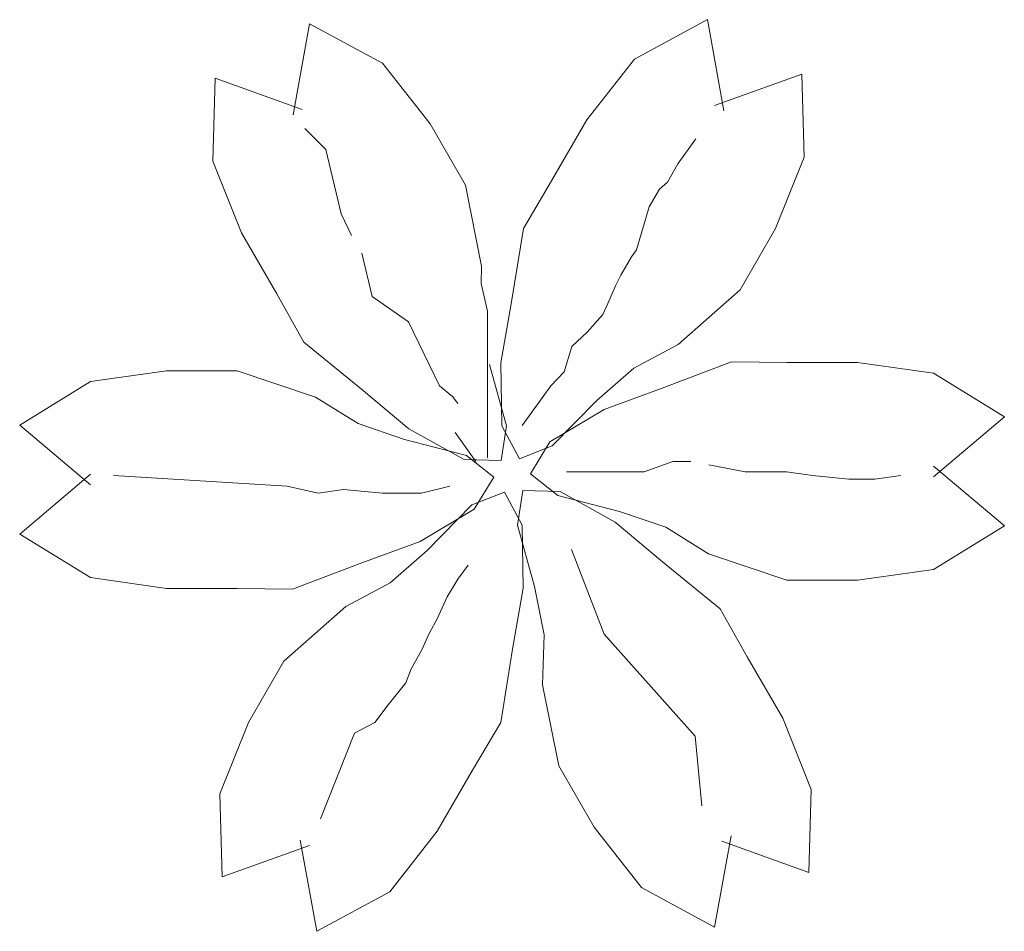
# Model space of a CAD drawing. Units: inches. Extents: x 1986 to 21484, y -1816 to 2016.
# Tile 85 of 85: x 21472.45 to 21483.96, y -1815.66 to -1805.01. Entities that reach past the tile are written whole.
import ezdxf

# ---------------------------------------------------------------- set-up
doc = ezdxf.new("R2010")
doc.units = ezdxf.units.IN
doc.layers.add('A-EQPM', color=9, linetype='Continuous', lineweight=18)

# ---------------------------------------------------------------- blocks, each defined once
blk = doc.blocks.new('ml')
for p, q in [((3455.34187, 1925.7691), (3455.34415, 1925.78173)), ((3455.34415, 1925.78173), (3455.35427, 1925.77626)), ((3455.39929, 1925.7823), (3455.38917, 1925.77683)), ((3455.40157, 1925.76967), (3455.39929, 1925.7823)), ((3455.35427, 1925.77626), (3455.36085, 1925.76787)), ((3455.38917, 1925.77683), (3455.38259, 1925.76844)), ((3455.40029, 1925.77041), (3455.41237, 1925.77475)), ((3455.41237, 1925.77475), (3455.4127, 1925.76325)), ((3455.33107, 1925.77418), (3455.33074, 1925.76268)), ((3455.34315, 1925.76984), (3455.33107, 1925.77418)), ((3455.36085, 1925.76787), (3455.36575, 1925.75939)), ((3455.38259, 1925.76844), (3455.37769, 1925.75996)), ((3455.34351, 1925.76724), (3455.3464, 1925.7643)), ((3455.39519, 1925.76234), (3455.39767, 1925.76577)), ((3455.3464, 1925.7643), (3455.34853, 1925.7554)), ((3455.33074, 1925.76268), (3455.33471, 1925.75278)), ((3455.39378, 1925.75981), (3455.39519, 1925.76234)), ((3455.4127, 1925.76325), (3455.40873, 1925.75335)), ((3455.37378, 1925.75338), (3455.37769, 1925.75996)), ((3455.39265, 1925.75883), (3455.39378, 1925.75981)), ((3455.36575, 1925.75939), (3455.368, 1925.74816)), ((3455.39124, 1925.75638), (3455.39265, 1925.75883)), ((3455.34853, 1925.7554), (3455.34995, 1925.75238)), ((3455.38946, 1925.75042), (3455.39124, 1925.75638)), ((3455.33471, 1925.75278), (3455.33961, 1925.7443)), ((3455.37215, 1925.7432), (3455.37378, 1925.75338)), ((3455.40873, 1925.75335), (3455.40383, 1925.74487)), ((3455.35142, 1925.74993), (3455.35284, 1925.74397)), ((3455.38876, 1925.74944), (3455.38946, 1925.75042)), ((3455.38728, 1925.74691), (3455.38876, 1925.74944)), ((3455.368, 1925.74816), (3455.36792, 1925.74576)), ((3455.38657, 1925.74544), (3455.38728, 1925.74691)), ((3455.36881, 1925.74193), (3455.36792, 1925.74576)), ((3455.38551, 1925.74299), (3455.38657, 1925.74544)), ((3455.40383, 1925.74487), (3455.39523, 1925.73731)), ((3455.34336, 1925.73762), (3455.33961, 1925.7443)), ((3455.35284, 1925.74397), (3455.35786, 1925.74046)), ((3455.37068, 1925.73477), (3455.37215, 1925.7432)), ((3455.36881, 1925.72158), (3455.36881, 1925.74193)), ((3455.3848, 1925.74144), (3455.38551, 1925.74299)), ((3455.35786, 1925.74046), (3455.36217, 1925.73156)), ((3455.38261, 1925.73899), (3455.3848, 1925.74144)), ((3455.38049, 1925.73703), (3455.38261, 1925.73899)), ((3455.35135, 1925.73112), (3455.34336, 1925.73762)), ((3455.37942, 1925.73352), (3455.38049, 1925.73703)), ((3455.39523, 1925.73731), (3455.3891, 1925.73403)), ((3455.39301, 1925.73123), (3455.40264, 1925.73491)), ((3455.40264, 1925.73491), (3455.41029, 1925.73481)), ((3455.31379, 1925.73216), (3455.32434, 1925.73367)), ((3455.32434, 1925.73367), (3455.33414, 1925.73367)), ((3455.33414, 1925.73367), (3455.34498, 1925.73001)), ((3455.36909, 1925.73453), (3455.37146, 1925.72601)), ((3455.37081, 1925.72603), (3455.37068, 1925.73477)), ((3455.3891, 1925.73403), (3455.38397, 1925.72955)), ((3455.42009, 1925.73481), (3455.41029, 1925.73481)), ((3455.43064, 1925.73331), (3455.42009, 1925.73481)), ((3455.37759, 1925.73156), (3455.37942, 1925.73352)), ((3455.44044, 1925.72728), (3455.43064, 1925.73331)), ((3455.30399, 1925.72613), (3455.31379, 1925.73216)), ((3455.35792, 1925.72563), (3455.35135, 1925.73112)), ((3455.36217, 1925.73156), (3455.36395, 1925.73009)), ((3455.37653, 1925.73009), (3455.37759, 1925.73156)), ((3455.38497, 1925.7283), (3455.39301, 1925.73123)), ((3455.34498, 1925.73001), (3455.35089, 1925.72634)), ((3455.36395, 1925.73009), (3455.36471, 1925.72911)), ((3455.37363, 1925.72609), (3455.37653, 1925.73009)), ((3455.38397, 1925.72955), (3455.37778, 1925.72324)), ((3455.37747, 1925.72381), (3455.38497, 1925.7283)), ((3455.43064, 1925.71898), (3455.44044, 1925.72728)), ((3455.31379, 1925.71784), (3455.30399, 1925.72613)), ((3455.35089, 1925.72634), (3455.35733, 1925.72413)), ((3455.36556, 1925.72138), (3455.35792, 1925.72563)), ((3455.37146, 1925.72601), (3455.37073, 1925.72123)), ((3455.37327, 1925.72147), (3455.37081, 1925.72603)), ((3455.35733, 1925.72413), (3455.36589, 1925.72193)), ((3455.36435, 1925.72509), (3455.36718, 1925.72109)), ((3455.37778, 1925.72324), (3455.37327, 1925.72147)), ((3455.37476, 1925.7194), (3455.37747, 1925.72381)), ((3455.37073, 1925.72123), (3455.36556, 1925.72138)), ((3455.36589, 1925.72193), (3455.36968, 1925.71891)), ((3455.39053, 1925.71964), (3455.39449, 1925.72111)), ((3455.39449, 1925.72111), (3455.39697, 1925.72111)), ((3455.39951, 1925.72062), (3455.40453, 1925.71964)), ((3455.43064, 1925.72046), (3455.44044, 1925.71217)), ((3455.31379, 1925.71932), (3455.30399, 1925.71103)), ((3455.31698, 1925.71915), (3455.34103, 1925.71768)), ((3455.36968, 1925.71891), (3455.36696, 1925.7145)), ((3455.37854, 1925.71638), (3455.37476, 1925.7194)), ((3455.37978, 1925.71964), (3455.38297, 1925.71964)), ((3455.38297, 1925.71964), (3455.39053, 1925.71964)), ((3455.40453, 1925.71964), (3455.41026, 1925.71964)), ((3455.41026, 1925.71964), (3455.41386, 1925.71915)), ((3455.41386, 1925.71915), (3455.41888, 1925.71866)), ((3455.41888, 1925.71866), (3455.42248, 1925.71866)), ((3455.42248, 1925.71866), (3455.42603, 1925.71915)), ((3455.34103, 1925.71768), (3455.34534, 1925.7167)), ((3455.34534, 1925.7167), (3455.34888, 1925.71719)), ((3455.34888, 1925.71719), (3455.35426, 1925.7167)), ((3455.35969, 1925.7167), (3455.36359, 1925.71768)), ((3455.35426, 1925.7167), (3455.35969, 1925.7167)), ((3455.36665, 1925.71507), (3455.37116, 1925.71683)), ((3455.37116, 1925.71683), (3455.37362, 1925.71227)), ((3455.37297, 1925.71229), (3455.3737, 1925.71707)), ((3455.3737, 1925.71707), (3455.37887, 1925.71693)), ((3455.3871, 1925.71417), (3455.37854, 1925.71638)), ((3455.37887, 1925.71693), (3455.38651, 1925.71267)), ((3455.36696, 1925.7145), (3455.35946, 1925.71001)), ((3455.36046, 1925.70875), (3455.36665, 1925.71507)), ((3455.39354, 1925.71197), (3455.3871, 1925.71417)), ((3455.37535, 1925.70377), (3455.37297, 1925.71229)), ((3455.37362, 1925.71227), (3455.37375, 1925.70353)), ((3455.38651, 1925.71267), (3455.39308, 1925.70719)), ((3455.39945, 1925.70829), (3455.39354, 1925.71197)), ((3455.44044, 1925.71217), (3455.43064, 1925.70614)), ((3455.30399, 1925.71103), (3455.31379, 1925.705)), ((3455.35946, 1925.71001), (3455.35142, 1925.70707)), ((3455.35533, 1925.70428), (3455.36046, 1925.70875)), ((3455.38044, 1925.70889), (3455.38496, 1925.69716)), ((3455.41029, 1925.70463), (3455.39945, 1925.70829)), ((3455.35142, 1925.70707), (3455.34179, 1925.7034)), ((3455.36471, 1925.70478), (3455.36613, 1925.70674)), ((3455.39308, 1925.70719), (3455.40107, 1925.70068)), ((3455.31379, 1925.705), (3455.32434, 1925.70349)), ((3455.43064, 1925.70614), (3455.42009, 1925.70463)), ((3455.3492, 1925.701), (3455.35533, 1925.70428)), ((3455.36324, 1925.70233), (3455.36471, 1925.70478)), ((3455.37375, 1925.70353), (3455.37228, 1925.6951)), ((3455.37666, 1925.69709), (3455.37535, 1925.70377)), ((3455.42009, 1925.70463), (3455.41029, 1925.70463)), ((3455.32434, 1925.70349), (3455.33414, 1925.70349)), ((3455.34179, 1925.7034), (3455.33414, 1925.70349)), ((3455.36182, 1925.69931), (3455.36324, 1925.70233)), ((3455.3406, 1925.69343), (3455.3492, 1925.701)), ((3455.40107, 1925.70068), (3455.40482, 1925.69401)), ((3455.36076, 1925.69735), (3455.36182, 1925.69931)), ((3455.35969, 1925.6949), (3455.36076, 1925.69735)), ((3455.37643, 1925.69014), (3455.37666, 1925.69709)), ((3455.38496, 1925.69716), (3455.3976, 1925.68302)), ((3455.35822, 1925.69237), (3455.35969, 1925.6949)), ((3455.37228, 1925.6951), (3455.37065, 1925.68493)), ((3455.40972, 1925.68552), (3455.40482, 1925.69401)), ((3455.3357, 1925.68495), (3455.3406, 1925.69343)), ((3455.35751, 1925.69041), (3455.35822, 1925.69237)), ((3455.35503, 1925.68739), (3455.35751, 1925.69041)), ((3455.37868, 1925.67892), (3455.37643, 1925.69014)), ((3455.35319, 1925.68494), (3455.35503, 1925.68739)), ((3455.33173, 1925.67506), (3455.3357, 1925.68495)), ((3455.35036, 1925.68347), (3455.35319, 1925.68494)), ((3455.37065, 1925.68493), (3455.36674, 1925.67834)), ((3455.41369, 1925.67563), (3455.40972, 1925.68552)), ((3455.34569, 1925.67156), (3455.35036, 1925.68347)), ((3455.3976, 1925.68302), (3455.39851, 1925.67339)), ((3455.36184, 1925.66986), (3455.36674, 1925.67834)), ((3455.38358, 1925.67043), (3455.37868, 1925.67892)), ((3455.33206, 1925.66356), (3455.33173, 1925.67506)), ((3455.41336, 1925.66413), (3455.41369, 1925.67563)), ((3455.35526, 1925.66147), (3455.36184, 1925.66986)), ((3455.39016, 1925.66205), (3455.38358, 1925.67043)), ((3455.34286, 1925.66864), (3455.34514, 1925.656)), ((3455.40256, 1925.66921), (3455.40028, 1925.65658)), ((3455.40128, 1925.66847), (3455.41336, 1925.66413)), ((3455.34414, 1925.6679), (3455.33206, 1925.66356)), ((3455.34514, 1925.656), (3455.35526, 1925.66147)), ((3455.40028, 1925.65658), (3455.39016, 1925.66205))]:
    blk.add_line(p, q)

msp = doc.modelspace()

# ---------------------------------------------------------------- block references
at = {"layer": 'A-EQPM', "xscale": 84.32671139547743, "yscale": 84.32671139547743, "zscale": 84.32671139547743}
msp.add_blockref('ml', (-269901.967, -164199.896), dxfattribs=at)

doc.saveas('drawing.dxf')
